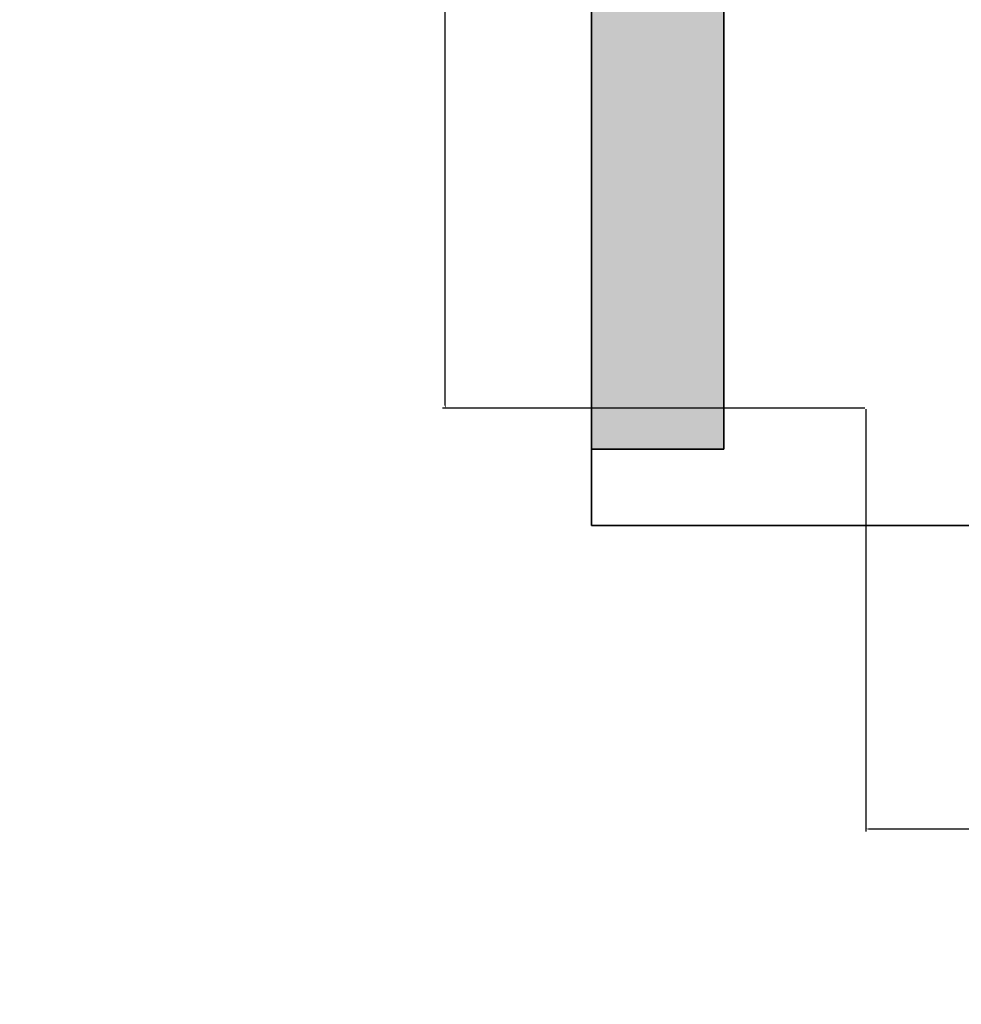
# Model space of a CAD drawing. Units: inches. Extents: x -4737294 to -4736756, y 1716389 to 1717040.
# Tile 1 of 25: x -4737254 to -4737190, y 1716424 to 1716491. Entities that reach past the tile are written whole.
import ezdxf

# ---------------------------------------------------------------- set-up
doc = ezdxf.new("R2010")
doc.units = ezdxf.units.IN
doc.header["$MEASUREMENT"] = 0
for name, color, linetype, lineweight in [('A-ANNO-DIMS', 2, 'Continuous', 18), ('A-WALL-PATT', 244, 'Continuous', 13), ('walls', 252, 'Continuous', 35)]:
    doc.layers.add(name, color=color, linetype=linetype, lineweight=lineweight)
doc.styles.get("Standard").update_dxf_attribs({"font": 'arial.ttf'})
doc.dimstyles.get("Standard").update_dxf_attribs({"dimtxt": 8, "dimasz": 0.18, "dimexe": 0.18, "dimexo": 0.0625, "dimgap": 0.09, "dimtad": 0, "dimtih": 1, "dimtoh": 1, "dimzin": 0, "dimdsep": 46, "dimlunit": 3, "dimtxsty": 'Standard', "dimcen": 0.09, "dimadec": 0, "dimazin": 0, "dimtfac": 1, "dimtofl": 0, "dimtmove": 0, "dimatfit": 3, "dimfxl": 1, "dimtolj": 1, "dimtzin": 0, "dimarcsym": 0})

# ---------------------------------------------------------------- blocks, each defined once
blk = doc.blocks.new('*D59')
at = {"layer": 'A-ANNO-DIMS', "color": 0, "lineweight": -2, "transparency": 16777216}
for p, q in [((-4737196.539, 1716655.661), (-4737225.279, 1716655.661)), ((-4737225.099, 1716655.481), (-4737225.099, 1716564.479)), ((-4737225.099, 1716465.024), (-4737225.099, 1716556.026)), ((-4737196.539, 1716464.844), (-4737225.279, 1716464.844))]:
    blk.add_line(p, q, dxfattribs=at)
at = {"layer": 'A-ANNO-DIMS', "color": 0, "transparency": 16777216}
for points in [[(-4737225.129, 1716655.481), (-4737225.069, 1716655.481), (-4737225.099, 1716655.661)], [(-4737225.129, 1716465.024), (-4737225.069, 1716465.024), (-4737225.099, 1716464.844)]]:
    blk.add_solid(points, dxfattribs=at)
at = {"layer": 'Defpoints', "color": 0, "transparency": 16777216}
for p in [(-4737196.476, 1716655.661), (-4737225.099, 1716464.844), (-4737196.476, 1716464.844)]:
    blk.add_point(p, dxfattribs=at)
at = {"layer": 'A-ANNO-DIMS', "color": 0, "transparency": 16777216, "insert": (-4737225.099, 1716560.253), "char_height": 8, "attachment_point": 5}
blk.add_mtext('\\A1;CAR 15\'-11"', dxfattribs=at)
blk = doc.blocks.new('*D60')
at = {"layer": 'A-ANNO-DIMS', "color": 0, "lineweight": -2, "transparency": 16777216}
for p, q in [((-4737196.476, 1716464.781), (-4737196.476, 1716436.041)), ((-4737102.951, 1716464.781), (-4737102.951, 1716436.041)), ((-4737196.296, 1716436.221), (-4737169.725, 1716436.221)), ((-4737103.131, 1716436.221), (-4737129.703, 1716436.221))]:
    blk.add_line(p, q, dxfattribs=at)
at = {"layer": 'A-ANNO-DIMS', "color": 0, "transparency": 16777216}
for points in [[(-4737196.296, 1716436.251), (-4737196.296, 1716436.191), (-4737196.476, 1716436.221)], [(-4737103.131, 1716436.251), (-4737103.131, 1716436.191), (-4737102.951, 1716436.221)]]:
    blk.add_solid(points, dxfattribs=at)
at = {"layer": 'Defpoints', "color": 0, "transparency": 16777216}
for p in [(-4737196.476, 1716464.844), (-4737102.951, 1716464.844), (-4737102.951, 1716436.221)]:
    blk.add_point(p, dxfattribs=at)
at = {"layer": 'A-ANNO-DIMS', "color": 0, "transparency": 16777216, "insert": (-4737149.714, 1716436.221), "char_height": 8, "attachment_point": 5}
blk.add_mtext('\\A1;7\'-9 1/2"', dxfattribs=at)

msp = doc.modelspace()

# ---------------------------------------------------------------- hatches: boundary and pattern name
at = {"layer": 'A-WALL-PATT'}
h = msp.add_hatch(color=256, dxfattribs=at)
h.dxf.hatch_style = 1
h.paths.add_polyline_path([(-4737206.144, 1716844.565), (-4737110.144, 1716844.565), (-4737110.144, 1716823.907), (-4737105.644, 1716823.907), (-4737105.644, 1716844.565), (-4737098.44, 1716844.565), (-4737098.44, 1716849.065), (-4737206.144, 1716849.065), (-4737206.144, 1716993.065), (-4736864.144, 1716993.065), (-4736864.144, 1716849.065), (-4736963.275, 1716849.065), (-4736994.446, 1716849.065), (-4736997.144, 1716849.065), (-4736997.144, 1716844.565), (-4736864.144, 1716844.565), (-4736864.144, 1716668.565), (-4736934.391, 1716668.565), (-4736934.391, 1716664.065), (-4736864.144, 1716664.065), (-4736864.144, 1716462.065), (-4736855.144, 1716462.065), (-4736855.144, 1717002.065), (-4737215.144, 1717002.065), (-4737215.144, 1716462.065), (-4737206.144, 1716462.065), (-4737206.144, 1716659.065), (-4737062.144, 1716659.065), (-4737062.144, 1716647.493), (-4737057.644, 1716647.493), (-4737057.644, 1716796.565), (-4737071.812, 1716796.565), (-4737071.812, 1716792.065), (-4737070.805, 1716792.065), (-4737062.144, 1716792.065), (-4737062.144, 1716668.065), (-4737206.144, 1716668.065), (-4737206.144, 1716792.065), (-4737093.784, 1716792.065), (-4737093.784, 1716796.565), (-4737206.144, 1716796.565)])

# ---------------------------------------------------------------- linework, layer by layer
at = {"layer": 'walls'}
for p, q in [((-4737215.144, 1716462.065), (-4737215.144, 1717002.065)), ((-4737206.144, 1716462.065), (-4737206.144, 1716659.065)), ((-4737215.144, 1716456.869), (-4737215.144, 1716467.261)), ((-4737206.144, 1716462.065), (-4737215.144, 1716462.065)), ((-4737215.144, 1716456.869), (-4737062.144, 1716456.869))]:
    msp.add_line(p, q, dxfattribs=at)

# ---------------------------------------------------------------- dimensions: what is measured, and where the dimension line sits
at = {"layer": 'A-ANNO-DIMS'}
dim = msp.add_linear_dim(base=(-4737225.099, 1716464.844), p1=(-4737196.476, 1716655.661), p2=(-4737196.476, 1716464.844), angle=270, text='CAR <>', dimstyle='Standard', override={"dimdec": 1, "dimlfac": 1, "dimrnd": 0, "dimzin": 1, "dimdsep": 46, "dimlunit": 4, "dimfrac": 2}, dxfattribs=at)
dim.commit()
dim.dimension.update_dxf_attribs({"geometry": '*D59', "text_midpoint": (-4737225.099, 1716560.253)})
dim = msp.add_linear_dim(base=(-4737102.951, 1716436.221), p1=(-4737196.476, 1716464.844), p2=(-4737102.951, 1716464.844), dimstyle='Standard', override={"dimdec": 1, "dimlfac": 1, "dimrnd": 0, "dimzin": 1, "dimdsep": 46, "dimlunit": 4, "dimfrac": 2}, dxfattribs=at)
dim.commit()
dim.dimension.update_dxf_attribs({"geometry": '*D60', "text_midpoint": (-4737149.714, 1716436.221)})

doc.saveas('drawing.dxf')
